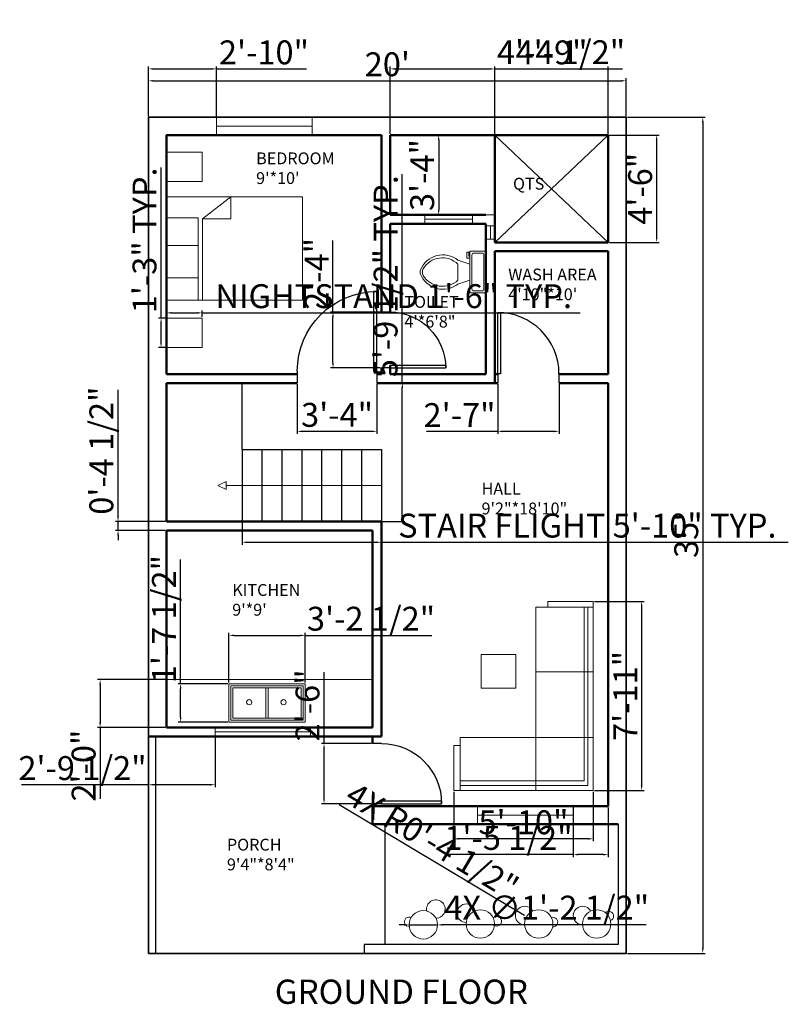
# Model space of a CAD drawing. Units: inches. Extents: x 2157 to 3060, y 2058 to 2553.
# Tile 1 of 2: x 2157 to 2543, y 2058 to 2553. Entities that reach past the tile are written whole.
import ezdxf

# ---------------------------------------------------------------- set-up
doc = ezdxf.new("R2010")
doc.units = ezdxf.units.IN
for name, color, linetype, lineweight in [('A-ANNO-DIMS', 2, 'Continuous', 18), ('A-ANNO-SYMB', 7, 'Continuous', 13), ('A-ANNO-TEXT', 7, 'Continuous', 35), ('A-AREA-IDEN', 7, 'Continuous', 18), ('A-FLOR', 7, 'Continuous', 25), ('A-FLOR-CASE', 32, 'Continuous', 20), ('A-FLOR-FIXT', 9, 'Continuous', 18), ('A-FLOR-STRS', 7, 'Continuous', 25), ('C-PROP', 7, 'Continuous', 35), ('DOOR', 2, 'Continuous', 25), ('FURNITURE', 32, 'Continuous', 18), ('L-PLNT', 3, 'Continuous', 18), ('WALL', 7, 'Continuous', 50), ('WINDOW', 130, 'Continuous', 18)]:
    doc.layers.add(name, color=color, linetype=linetype, lineweight=lineweight)
doc.styles.get("Standard").update_dxf_attribs({"font": 'arial.ttf'})
doc.dimstyles.new('ISO-25', dxfattribs={"dimtxt": 12, "dimasz": 2.5, "dimexe": 1.25, "dimexo": 0.625, "dimtad": 1, "dimdec": 0, "dimlunit": 4, "dimtxsty": 'Standard', "dimcen": 2.5, "dimadec": 0, "dimazin": 0, "dimtfac": 1, "dimtdec": 0, "dimtmove": 0, "dimatfit": 3, "dimfxl": 1, "dimarcsym": 0})

# ---------------------------------------------------------------- blocks, each defined once
blk = doc.blocks.new('*U2')
for p, q in [((0, 0), (0, -6)), ((40, 0), (40, -6))]:
    blk.add_line(p, q)
blk.add_lwpolyline([(0, 0), (0, 40), (1.75, 40), (1.75, 0)], close=True)
blk.add_arc((0, 0), 40, 0, 90)
blk = doc.blocks.new('*U4')
for p, q in [((9.5, -6), (9.5, -2)), ((-10, -8.5), (-8, -8.5)), ((-10, -9.5), (-10, -8.5)), ((-7, -9.5), (-10, -9.5)), ((-8, -8.5), (-8, -8)), ((-7, -8), (-7, -9.5)), ((-4, -8), (-6, -14)), ((4, -8), (6, -14)), ((4, -14), (-4, -14))]:
    blk.add_line(p, q)
blk.add_lwpolyline([(10.5, -8), (10.5, 0), (-10.5, 0), (-10.5, -8)], close=True)
for points in [[(-9.5, -2), (-9.5, -6)], [(8.5, -1), (-8.5, -1)], [(-8.5, -7), (8.5, -7)]]:
    blk.add_lwpolyline(points)
for centre, radius, start, end in [((-8.62, -1.88), 0.884, 81.8699, 188.1301), ((8.62, -1.88), 0.884, 351.8699, 98.1301), ((-8.62, -6.12), 0.884, 171.8699, 278.1301), ((8.62, -6.12), 0.884, 261.8699, 8.1301), ((3.52, -21.58), 12.17, 141.4691, 247.9714), ((4.2, -21.82), 11.33, 136.3677, 238.9468), ((-3.52, -21.58), 12.17, 292.0284, 38.5307), ((-4.2, -21.82), 11.33, 301.053, 43.6321), ((0, -27.88), 4, 245.7318, 294.2682), ((0, -29), 4, 254.8605, 285.1395)]:
    blk.add_arc(centre, radius, start, end)
blk = doc.blocks.new('*D5')
at = {"layer": 'A-ANNO-DIMS', "color": 0, "lineweight": -2, "transparency": 16777216}
for p, q in [((2222.04, 2504.59), (2222.04, 2523.53)), ((2462.04, 2504.59), (2462.04, 2523.53)), ((2224.54, 2522.28), (2459.54, 2522.28))]:
    blk.add_line(p, q, dxfattribs=at)
at = {"layer": 'A-ANNO-DIMS', "color": 0, "transparency": 16777216}
for points in [[(2224.54, 2522.7), (2224.54, 2521.86), (2222.04, 2522.28)], [(2459.54, 2522.7), (2459.54, 2521.86), (2462.04, 2522.28)]]:
    blk.add_solid(points, dxfattribs=at)
at = {"layer": 'Defpoints', "color": 0, "transparency": 16777216}
for p in [(2462.04, 2522.28), (2222.04, 2503.96), (2462.04, 2503.96)]:
    blk.add_point(p, dxfattribs=at)
at = {"layer": 'A-ANNO-DIMS', "color": 0, "transparency": 16777216, "insert": (2342.04, 2529.03), "char_height": 12, "attachment_point": 5}
blk.add_mtext("20'", dxfattribs=at)
blk = doc.blocks.new('*D6')
at = {"layer": 'A-ANNO-DIMS', "color": 0, "lineweight": -2, "transparency": 16777216}
for p, q in [((2462.67, 2503.96), (2501.77, 2503.96)), ((2500.52, 2501.46), (2500.52, 2086.46)), ((2462.67, 2083.96), (2501.77, 2083.96))]:
    blk.add_line(p, q, dxfattribs=at)
at = {"layer": 'A-ANNO-DIMS', "color": 0, "transparency": 16777216}
for points in [[(2500.1, 2501.46), (2500.94, 2501.46), (2500.52, 2503.96)], [(2500.1, 2086.46), (2500.94, 2086.46), (2500.52, 2083.96)]]:
    blk.add_solid(points, dxfattribs=at)
at = {"layer": 'Defpoints', "color": 0, "transparency": 16777216}
for p in [(2462.04, 2503.96), (2462.04, 2083.96), (2500.52, 2083.96)]:
    blk.add_point(p, dxfattribs=at)
at = {"layer": 'A-ANNO-DIMS', "color": 0, "transparency": 16777216, "insert": (2493.76, 2293.96), "char_height": 12, "attachment_point": 5, "rotation": 90}
blk.add_mtext("35'", dxfattribs=at)
blk = doc.blocks.new('BED-DOUBLE')
for p, q in [((18.2, 40.88), (32.33, 51.9)), ((32.33, 40.88), (32.33, 51.9)), ((18.2, 0), (18.2, 40.88)), ((18.2, 40.88), (32.33, 40.88)), ((0, 27.39), (15.88, 27.39)), ((0, 11.16), (15.88, 11.16))]:
    blk.add_line(p, q)
for points in [[(0, 0), (68.32, 0), (68.32, 51.9), (0, 51.9)], [(0, 0), (15.88, 0), (15.88, 41.3), (0, 41.3)]]:
    blk.add_lwpolyline(points, close=True)
blk = doc.blocks.new('NIGHTSTAND')
blk.add_lwpolyline([(0, 0), (17.99, 0), (17.99, 14.76), (0, 14.76)], close=True)
blk = doc.blocks.new('STAIR-FLIGHT')
for p, q in [((0, 36.14), (0, 69.5)), ((0, 36.14), (70, 36.14)), ((0, 36.14), (0, 0)), ((0, 36.14), (0, 0)), ((0, 36.14), (0, 0)), ((0, 36.14), (0, 0)), ((10, 36.14), (10, 0)), ((10, 36.14), (10, 0)), ((10, 36.14), (10, 0)), ((10, 36.14), (10, 0)), ((20, 36.14), (20, 0)), ((30, 36.14), (30, 0)), ((30, 36.14), (30, 0)), ((30, 36.14), (30, 0)), ((30, 36.14), (30, 0)), ((40, 36.14), (40, 0)), ((50, 36.14), (50, 0)), ((50, 36.14), (50, 0)), ((50, 36.14), (50, 0)), ((50, 36.14), (50, 0)), ((60, 36.14), (60, 0)), ((70, 36.14), (70, 0))]:
    blk.add_line(p, q)
blk = doc.blocks.new('STAIR-DIRECTION')
for p, q in [((4.17, 4), (0, 2)), ((0, 2), (4.17, 0)), ((4.17, 0), (4.17, 4)), ((82.21, 2), (4.17, 2)), ((4.17, 2), (4.17, 0))]:
    blk.add_line(p, q)
blk = doc.blocks.new('WIN-48IN-EXT')
for p, q in [((0, 4.5), (0, 9)), ((48, 4.5), (48, 9)), ((0, 4.5), (0, 0)), ((0, 4.5), (48, 4.5)), ((48, 4.5), (48, 0))]:
    blk.add_line(p, q)
blk = doc.blocks.new('OPEN-TO-SKY-MARK')
for p, q in [((57, 53.82), (0, 0)), ((57, 0), (0, 53.82))]:
    blk.add_line(p, q)
blk = doc.blocks.new('*D15')
at = {"layer": 'A-ANNO-DIMS', "color": 0, "lineweight": -2, "transparency": 16777216}
for p, q in [((2231.04, 2403.64), (2231.04, 2406.96)), ((2233.54, 2405.71), (2246.53, 2405.71)), ((2249.03, 2403.64), (2249.03, 2406.96)), ((2249.03, 2405.71), (2438.97, 2405.71))]:
    blk.add_line(p, q, dxfattribs=at)
at = {"layer": 'A-ANNO-DIMS', "color": 0, "transparency": 16777216}
for points in [[(2233.54, 2406.13), (2233.54, 2405.3), (2231.04, 2405.71)], [(2246.53, 2406.13), (2246.53, 2405.3), (2249.03, 2405.71)]]:
    blk.add_solid(points, dxfattribs=at)
at = {"layer": 'Defpoints', "color": 0, "transparency": 16777216}
for p in [(2249.03, 2405.71), (2231.04, 2403.02), (2249.03, 2403.02)]:
    blk.add_point(p, dxfattribs=at)
at = {"layer": 'A-ANNO-DIMS', "color": 0, "transparency": 16777216, "insert": (2345.25, 2412.54), "char_height": 12, "attachment_point": 5}
blk.add_mtext('NIGHTSTAND 1\'-6" TYP.', dxfattribs=at)
blk = doc.blocks.new('*D16')
at = {"layer": 'A-ANNO-DIMS', "color": 0, "lineweight": -2, "transparency": 16777216}
for p, q in [((2228.35, 2403.02), (2228.35, 2478.78)), ((2230.42, 2403.02), (2227.1, 2403.02)), ((2228.35, 2390.76), (2228.35, 2400.52)), ((2230.42, 2388.26), (2227.1, 2388.26))]:
    blk.add_line(p, q, dxfattribs=at)
at = {"layer": 'A-ANNO-DIMS', "color": 0, "transparency": 16777216}
for points in [[(2227.93, 2400.52), (2228.76, 2400.52), (2228.35, 2403.02)], [(2227.93, 2390.76), (2228.76, 2390.76), (2228.35, 2388.26)]]:
    blk.add_solid(points, dxfattribs=at)
at = {"layer": 'Defpoints', "color": 0, "transparency": 16777216}
for p in [(2228.35, 2403.02), (2231.04, 2403.02), (2231.04, 2388.26)]:
    blk.add_point(p, dxfattribs=at)
at = {"layer": 'A-ANNO-DIMS', "color": 0, "transparency": 16777216, "insert": (2221.59, 2442.15), "char_height": 12, "attachment_point": 5, "rotation": 90}
blk.add_mtext('1\'-3" TYP.', dxfattribs=at)
blk = doc.blocks.new('*D21')
at = {"layer": 'A-ANNO-DIMS', "color": 0, "lineweight": -2, "transparency": 16777216}
for p, q in [((2269.04, 2300.34), (2269.04, 2289.21)), ((2339.04, 2300.34), (2339.04, 2289.21)), ((2271.54, 2290.46), (2336.54, 2290.46)), ((2339.04, 2290.46), (2543.5, 2290.46))]:
    blk.add_line(p, q, dxfattribs=at)
at = {"layer": 'A-ANNO-DIMS', "color": 0, "transparency": 16777216}
for points in [[(2271.54, 2290.88), (2271.54, 2290.05), (2269.04, 2290.46)], [(2336.54, 2290.88), (2336.54, 2290.05), (2339.04, 2290.46)]]:
    blk.add_solid(points, dxfattribs=at)
at = {"layer": 'Defpoints', "color": 0, "transparency": 16777216}
for p in [(2269.04, 2300.96), (2339.04, 2300.96), (2339.04, 2290.46)]:
    blk.add_point(p, dxfattribs=at)
at = {"layer": 'A-ANNO-DIMS', "color": 0, "transparency": 16777216, "insert": (2442.52, 2297.29), "char_height": 12, "attachment_point": 5}
blk.add_mtext('STAIR FLIGHT 5\'-10" TYP.', dxfattribs=at)
blk = doc.blocks.new('*D22')
at = {"layer": 'A-ANNO-DIMS', "color": 0, "lineweight": -2, "transparency": 16777216}
for p, q in [((2349.54, 2370.46), (2349.54, 2475.32)), ((2339.67, 2370.46), (2350.79, 2370.46)), ((2349.54, 2303.46), (2349.54, 2367.96)), ((2339.67, 2300.96), (2350.79, 2300.96))]:
    blk.add_line(p, q, dxfattribs=at)
at = {"layer": 'A-ANNO-DIMS', "color": 0, "transparency": 16777216}
for points in [[(2349.13, 2367.96), (2349.96, 2367.96), (2349.54, 2370.46)], [(2349.13, 2303.46), (2349.96, 2303.46), (2349.54, 2300.96)]]:
    blk.add_solid(points, dxfattribs=at)
at = {"layer": 'Defpoints', "color": 0, "transparency": 16777216}
for p in [(2339.04, 2370.46), (2349.54, 2370.46), (2339.04, 2300.96)]:
    blk.add_point(p, dxfattribs=at)
at = {"layer": 'A-ANNO-DIMS', "color": 0, "transparency": 16777216, "insert": (2342.71, 2424.14), "char_height": 12, "attachment_point": 5, "rotation": 90}
blk.add_mtext('5\'-9 1/2" TYP.', dxfattribs=at)
blk = doc.blocks.new('*D23')
at = {"layer": 'A-ANNO-DIMS', "color": 0, "lineweight": -2, "transparency": 16777216}
for p, q in [((2396.04, 2495.59), (2396.04, 2529.51)), ((2398.54, 2528.26), (2450.54, 2528.26)), ((2453.04, 2495.59), (2453.04, 2529.51))]:
    blk.add_line(p, q, dxfattribs=at)
at = {"layer": 'A-ANNO-DIMS', "color": 0, "transparency": 16777216}
for points in [[(2398.54, 2528.68), (2398.54, 2527.85), (2396.04, 2528.26)], [(2450.54, 2528.68), (2450.54, 2527.85), (2453.04, 2528.26)]]:
    blk.add_solid(points, dxfattribs=at)
at = {"layer": 'Defpoints', "color": 0, "transparency": 16777216}
for p in [(2453.04, 2528.26), (2396.04, 2494.96), (2453.04, 2494.96)]:
    blk.add_point(p, dxfattribs=at)
at = {"layer": 'A-ANNO-DIMS', "color": 0, "transparency": 16777216, "insert": (2424.54, 2535.01), "char_height": 12, "attachment_point": 5}
blk.add_mtext('4\'-9"', dxfattribs=at)
blk = doc.blocks.new('*D24')
at = {"layer": 'A-ANNO-DIMS', "color": 0, "lineweight": -2, "transparency": 16777216}
for p, q in [((2453.67, 2494.96), (2478.59, 2494.96)), ((2477.34, 2492.46), (2477.34, 2443.64)), ((2453.67, 2441.14), (2478.59, 2441.14))]:
    blk.add_line(p, q, dxfattribs=at)
at = {"layer": 'A-ANNO-DIMS', "color": 0, "transparency": 16777216}
for points in [[(2476.93, 2492.46), (2477.76, 2492.46), (2477.34, 2494.96)], [(2476.93, 2443.64), (2477.76, 2443.64), (2477.34, 2441.14)]]:
    blk.add_solid(points, dxfattribs=at)
at = {"layer": 'Defpoints', "color": 0, "transparency": 16777216}
for p in [(2453.04, 2494.96), (2453.04, 2441.14), (2477.34, 2441.14)]:
    blk.add_point(p, dxfattribs=at)
at = {"layer": 'A-ANNO-DIMS', "color": 0, "transparency": 16777216, "insert": (2470.59, 2468.05), "char_height": 12, "attachment_point": 5, "rotation": 90}
blk.add_mtext('4\'-6"', dxfattribs=at)
blk = doc.blocks.new('*D27')
at = {"layer": 'A-ANNO-DIMS', "color": 0, "lineweight": -2, "transparency": 16777216}
for p, q in [((2310.24, 2189.36), (2310.24, 2225.21)), ((2333.92, 2189.36), (2308.99, 2189.36)), ((2310.24, 2161.64), (2310.24, 2186.86)), ((2333.92, 2159.14), (2308.99, 2159.14))]:
    blk.add_line(p, q, dxfattribs=at)
at = {"layer": 'A-ANNO-DIMS', "color": 0, "transparency": 16777216}
for points in [[(2309.83, 2186.86), (2310.66, 2186.86), (2310.24, 2189.36)], [(2309.83, 2161.64), (2310.66, 2161.64), (2310.24, 2159.14)]]:
    blk.add_solid(points, dxfattribs=at)
at = {"layer": 'Defpoints', "color": 0, "transparency": 16777216}
for p in [(2310.24, 2189.36), (2334.54, 2189.36), (2334.54, 2159.14)]:
    blk.add_point(p, dxfattribs=at)
at = {"layer": 'A-ANNO-DIMS', "color": 0, "transparency": 16777216, "insert": (2303.49, 2208.54), "char_height": 12, "attachment_point": 5, "rotation": 90}
blk.add_mtext('2\'-6"', dxfattribs=at)
blk = doc.blocks.new('*D29')
at = {"layer": 'A-ANNO-DIMS', "color": 0, "lineweight": -2, "transparency": 16777216}
for p, q in [((2230.42, 2221.46), (2196.49, 2221.46)), ((2197.74, 2218.96), (2197.74, 2199.96)), ((2230.42, 2197.46), (2196.49, 2197.46)), ((2197.74, 2197.46), (2197.74, 2161.61))]:
    blk.add_line(p, q, dxfattribs=at)
at = {"layer": 'A-ANNO-DIMS', "color": 0, "transparency": 16777216}
for points in [[(2197.33, 2218.96), (2198.16, 2218.96), (2197.74, 2221.46)], [(2197.33, 2199.96), (2198.16, 2199.96), (2197.74, 2197.46)]]:
    blk.add_solid(points, dxfattribs=at)
at = {"layer": 'Defpoints', "color": 0, "transparency": 16777216}
for p in [(2231.04, 2221.46), (2197.74, 2197.46), (2231.04, 2197.46)]:
    blk.add_point(p, dxfattribs=at)
at = {"layer": 'A-ANNO-DIMS', "color": 0, "transparency": 16777216, "insert": (2190.99, 2178.28), "char_height": 12, "attachment_point": 5, "rotation": 90}
blk.add_mtext('2\'-0"', dxfattribs=at)
blk = doc.blocks.new('*D30')
at = {"layer": 'A-ANNO-DIMS', "color": 0, "lineweight": -2, "transparency": 16777216}
for p, q in [((2222.04, 2504.59), (2222.04, 2529.51)), ((2224.54, 2528.26), (2253.72, 2528.26)), ((2256.22, 2504.59), (2256.22, 2529.51)), ((2256.22, 2528.26), (2301.4, 2528.26))]:
    blk.add_line(p, q, dxfattribs=at)
at = {"layer": 'A-ANNO-DIMS', "color": 0, "transparency": 16777216}
for points in [[(2224.54, 2528.68), (2224.54, 2527.85), (2222.04, 2528.26)], [(2253.72, 2528.68), (2253.72, 2527.85), (2256.22, 2528.26)]]:
    blk.add_solid(points, dxfattribs=at)
at = {"layer": 'Defpoints', "color": 0, "transparency": 16777216}
for p in [(2256.22, 2528.26), (2222.04, 2503.96), (2256.22, 2503.96)]:
    blk.add_point(p, dxfattribs=at)
at = {"layer": 'A-ANNO-DIMS', "color": 0, "transparency": 16777216, "insert": (2280.06, 2535.01), "char_height": 12, "attachment_point": 5}
blk.add_mtext('2\'-10"', dxfattribs=at)
blk = doc.blocks.new('*D32')
at = {"layer": 'A-ANNO-DIMS', "color": 0, "lineweight": -2, "transparency": 16777216}
for p, q in [((2222.04, 2192.34), (2222.04, 2167.41)), ((2255.49, 2192.34), (2255.49, 2167.41)), ((2222.04, 2168.66), (2158.23, 2168.66)), ((2252.99, 2168.66), (2224.54, 2168.66))]:
    blk.add_line(p, q, dxfattribs=at)
at = {"layer": 'A-ANNO-DIMS', "color": 0, "transparency": 16777216}
for points in [[(2224.54, 2169.08), (2224.54, 2168.25), (2222.04, 2168.66)], [(2252.99, 2169.08), (2252.99, 2168.25), (2255.49, 2168.66)]]:
    blk.add_solid(points, dxfattribs=at)
at = {"layer": 'Defpoints', "color": 0, "transparency": 16777216}
for p in [(2222.04, 2192.96), (2255.49, 2192.96), (2222.04, 2168.66)]:
    blk.add_point(p, dxfattribs=at)
at = {"layer": 'A-ANNO-DIMS', "color": 0, "transparency": 16777216, "insert": (2188.89, 2175.49), "char_height": 12, "attachment_point": 5}
blk.add_mtext('2\'-9 1/2"', dxfattribs=at)
blk = doc.blocks.new('*D33')
at = {"layer": 'A-ANNO-DIMS', "color": 0, "lineweight": -2, "transparency": 16777216}
for p, q in [((2435.4, 2157.26), (2435.4, 2132.33)), ((2453.04, 2157.26), (2453.04, 2132.33)), ((2435.4, 2133.58), (2372.92, 2133.58)), ((2450.54, 2133.58), (2437.9, 2133.58))]:
    blk.add_line(p, q, dxfattribs=at)
at = {"layer": 'A-ANNO-DIMS', "color": 0, "transparency": 16777216}
for points in [[(2437.9, 2134), (2437.9, 2133.16), (2435.4, 2133.58)], [(2450.54, 2134), (2450.54, 2133.16), (2453.04, 2133.58)]]:
    blk.add_solid(points, dxfattribs=at)
at = {"layer": 'Defpoints', "color": 0, "transparency": 16777216}
for p in [(2435.4, 2157.88), (2453.04, 2157.88), (2435.4, 2133.58)]:
    blk.add_point(p, dxfattribs=at)
at = {"layer": 'A-ANNO-DIMS', "color": 0, "transparency": 16777216, "insert": (2402.91, 2140.41), "char_height": 12, "attachment_point": 5}
blk.add_mtext('1\'-5 1/2"', dxfattribs=at)
blk = doc.blocks.new('*D36')
at = {"layer": 'A-ANNO-DIMS', "color": 0, "lineweight": -2, "transparency": 16777216}
for p, q in [((2296.79, 2369.84), (2296.79, 2344.91)), ((2336.79, 2369.84), (2336.79, 2344.91)), ((2334.29, 2346.16), (2299.29, 2346.16))]:
    blk.add_line(p, q, dxfattribs=at)
at = {"layer": 'A-ANNO-DIMS', "color": 0, "transparency": 16777216}
for points in [[(2299.29, 2346.58), (2299.29, 2345.75), (2296.79, 2346.16)], [(2334.29, 2346.58), (2334.29, 2345.75), (2336.79, 2346.16)]]:
    blk.add_solid(points, dxfattribs=at)
at = {"layer": 'Defpoints', "color": 0, "transparency": 16777216}
for p in [(2296.79, 2370.46), (2336.79, 2370.46), (2296.79, 2346.16)]:
    blk.add_point(p, dxfattribs=at)
at = {"layer": 'A-ANNO-DIMS', "color": 0, "transparency": 16777216, "insert": (2316.79, 2352.92), "char_height": 12, "attachment_point": 5}
blk.add_mtext('3\'-4"', dxfattribs=at)
blk = doc.blocks.new('*D37')
at = {"layer": 'A-ANNO-DIMS', "color": 0, "lineweight": -2, "transparency": 16777216}
for p, q in [((2397.49, 2369.84), (2397.49, 2344.91)), ((2428.29, 2369.84), (2428.29, 2344.91)), ((2397.49, 2346.16), (2361.64, 2346.16)), ((2425.79, 2346.16), (2399.99, 2346.16))]:
    blk.add_line(p, q, dxfattribs=at)
at = {"layer": 'A-ANNO-DIMS', "color": 0, "transparency": 16777216}
for points in [[(2399.99, 2346.58), (2399.99, 2345.75), (2397.49, 2346.16)], [(2425.79, 2346.58), (2425.79, 2345.75), (2428.29, 2346.16)]]:
    blk.add_solid(points, dxfattribs=at)
at = {"layer": 'Defpoints', "color": 0, "transparency": 16777216}
for p in [(2397.49, 2370.46), (2428.29, 2370.46), (2397.49, 2346.16)]:
    blk.add_point(p, dxfattribs=at)
at = {"layer": 'A-ANNO-DIMS', "color": 0, "transparency": 16777216, "insert": (2378.31, 2352.81), "char_height": 12, "attachment_point": 5}
blk.add_mtext('2\'-7"', dxfattribs=at)
blk = doc.blocks.new('*D38')
at = {"layer": 'A-ANNO-DIMS', "color": 0, "lineweight": -2, "transparency": 16777216}
for p, q in [((2314.74, 2406.14), (2314.74, 2441.99)), ((2338.42, 2406.14), (2313.49, 2406.14)), ((2314.74, 2380.53), (2314.74, 2403.64)), ((2338.42, 2378.03), (2313.49, 2378.03))]:
    blk.add_line(p, q, dxfattribs=at)
at = {"layer": 'A-ANNO-DIMS', "color": 0, "transparency": 16777216}
for points in [[(2314.33, 2403.64), (2315.16, 2403.64), (2314.74, 2406.14)], [(2314.33, 2380.53), (2315.16, 2380.53), (2314.74, 2378.03)]]:
    blk.add_solid(points, dxfattribs=at)
at = {"layer": 'Defpoints', "color": 0, "transparency": 16777216}
for p in [(2314.74, 2406.14), (2339.04, 2406.14), (2339.04, 2378.03)]:
    blk.add_point(p, dxfattribs=at)
at = {"layer": 'A-ANNO-DIMS', "color": 0, "transparency": 16777216, "insert": (2308.09, 2425.31), "char_height": 12, "attachment_point": 5, "rotation": 90}
blk.add_mtext('2\'-4"', dxfattribs=at)
blk = doc.blocks.new('*D41')
at = {"layer": 'A-ANNO-DIMS', "color": 0, "lineweight": -2, "transparency": 16777216}
for p, q in [((2375.38, 2165.16), (2375.38, 2140.24)), ((2445.5, 2165.16), (2445.5, 2140.24)), ((2443, 2141.49), (2377.88, 2141.49))]:
    blk.add_line(p, q, dxfattribs=at)
at = {"layer": 'A-ANNO-DIMS', "color": 0, "transparency": 16777216}
for points in [[(2377.88, 2141.91), (2377.88, 2141.07), (2375.38, 2141.49)], [(2443, 2141.91), (2443, 2141.07), (2445.5, 2141.49)]]:
    blk.add_solid(points, dxfattribs=at)
at = {"layer": 'Defpoints', "color": 0, "transparency": 16777216}
for p in [(2375.38, 2165.79), (2445.5, 2165.79), (2375.38, 2141.49)]:
    blk.add_point(p, dxfattribs=at)
at = {"layer": 'A-ANNO-DIMS', "color": 0, "transparency": 16777216, "insert": (2410.44, 2148.24), "char_height": 12, "attachment_point": 5}
blk.add_mtext('5\'-10"', dxfattribs=at)
blk = doc.blocks.new('*D42')
at = {"layer": 'A-ANNO-DIMS', "color": 0, "lineweight": -2, "transparency": 16777216}
for p, q in [((2446.13, 2260.8), (2471.05, 2260.8)), ((2469.8, 2258.3), (2469.8, 2168.29)), ((2446.13, 2165.79), (2471.05, 2165.79))]:
    blk.add_line(p, q, dxfattribs=at)
at = {"layer": 'A-ANNO-DIMS', "color": 0, "transparency": 16777216}
for points in [[(2469.39, 2258.3), (2470.22, 2258.3), (2469.8, 2260.8)], [(2469.39, 2168.29), (2470.22, 2168.29), (2469.8, 2165.79)]]:
    blk.add_solid(points, dxfattribs=at)
at = {"layer": 'Defpoints', "color": 0, "transparency": 16777216}
for p in [(2445.5, 2260.8), (2445.5, 2165.79), (2469.8, 2165.79)]:
    blk.add_point(p, dxfattribs=at)
at = {"layer": 'A-ANNO-DIMS', "color": 0, "transparency": 16777216, "insert": (2463.15, 2213.29), "char_height": 12, "attachment_point": 5, "rotation": 90}
blk.add_mtext('7\'-11"', dxfattribs=at)
blk = doc.blocks.new('*D43')
at = {"layer": 'A-ANNO-DIMS', "color": 0, "lineweight": -2, "transparency": 16777216}
for p, q in [((2262.49, 2220.01), (2262.49, 2244.94)), ((2264.99, 2243.69), (2298.31, 2243.69)), ((2300.81, 2220.01), (2300.81, 2244.94)), ((2300.81, 2243.69), (2364.41, 2243.69))]:
    blk.add_line(p, q, dxfattribs=at)
at = {"layer": 'A-ANNO-DIMS', "color": 0, "transparency": 16777216}
for points in [[(2264.99, 2244.1), (2264.99, 2243.27), (2262.49, 2243.69)], [(2298.31, 2244.1), (2298.31, 2243.27), (2300.81, 2243.69)]]:
    blk.add_solid(points, dxfattribs=at)
at = {"layer": 'Defpoints', "color": 0, "transparency": 16777216}
for p in [(2300.81, 2243.69), (2262.49, 2219.39), (2300.81, 2219.39)]:
    blk.add_point(p, dxfattribs=at)
at = {"layer": 'A-ANNO-DIMS', "color": 0, "transparency": 16777216, "insert": (2333.86, 2250.52), "char_height": 12, "attachment_point": 5}
blk.add_mtext('3\'-2 1/2"', dxfattribs=at)
blk = doc.blocks.new('*D44')
at = {"layer": 'A-ANNO-DIMS', "color": 0, "lineweight": -2, "transparency": 16777216}
for p, q in [((2238.19, 2219.39), (2238.19, 2281.87)), ((2261.87, 2219.39), (2236.94, 2219.39)), ((2238.19, 2202.61), (2238.19, 2216.89)), ((2261.87, 2200.11), (2236.94, 2200.11))]:
    blk.add_line(p, q, dxfattribs=at)
at = {"layer": 'A-ANNO-DIMS', "color": 0, "transparency": 16777216}
for points in [[(2237.78, 2216.89), (2238.61, 2216.89), (2238.19, 2219.39)], [(2237.78, 2202.61), (2238.61, 2202.61), (2238.19, 2200.11)]]:
    blk.add_solid(points, dxfattribs=at)
at = {"layer": 'Defpoints', "color": 0, "transparency": 16777216}
for p in [(2238.19, 2219.39), (2262.49, 2219.39), (2262.49, 2200.11)]:
    blk.add_point(p, dxfattribs=at)
at = {"layer": 'A-ANNO-DIMS', "color": 0, "transparency": 16777216, "insert": (2231.36, 2251.88), "char_height": 12, "attachment_point": 5, "rotation": 90}
blk.add_mtext('1\'-7 1/2"', dxfattribs=at)
blk = doc.blocks.new('*D47')
at = {"layer": 'A-ANNO-DIMS', "color": 0, "lineweight": -2, "transparency": 16777216}
for p, q in [((2343.54, 2495.59), (2343.54, 2529.51)), ((2346.04, 2528.26), (2393.54, 2528.26)), ((2396.04, 2495.59), (2396.04, 2529.51)), ((2396.04, 2528.26), (2460.14, 2528.26))]:
    blk.add_line(p, q, dxfattribs=at)
at = {"layer": 'A-ANNO-DIMS', "color": 0, "transparency": 16777216}
for points in [[(2346.04, 2528.68), (2346.04, 2527.85), (2343.54, 2528.26)], [(2393.54, 2528.68), (2393.54, 2527.85), (2396.04, 2528.26)]]:
    blk.add_solid(points, dxfattribs=at)
at = {"layer": 'Defpoints', "color": 0, "transparency": 16777216}
for p in [(2396.04, 2528.26), (2343.54, 2494.96), (2396.04, 2494.96)]:
    blk.add_point(p, dxfattribs=at)
at = {"layer": 'A-ANNO-DIMS', "color": 0, "transparency": 16777216, "insert": (2429.34, 2535.09), "char_height": 12, "attachment_point": 5}
blk.add_mtext('4\'-4 1/2"', dxfattribs=at)
blk = doc.blocks.new('*D48')
at = {"layer": 'A-ANNO-DIMS', "color": 0, "lineweight": -2, "transparency": 16777216}
for p, q in [((2344.17, 2494.96), (2369.09, 2494.96)), ((2367.84, 2492.46), (2367.84, 2457.46)), ((2344.17, 2454.96), (2369.09, 2454.96))]:
    blk.add_line(p, q, dxfattribs=at)
at = {"layer": 'A-ANNO-DIMS', "color": 0, "transparency": 16777216}
for points in [[(2367.43, 2492.46), (2368.26, 2492.46), (2367.84, 2494.96)], [(2367.43, 2457.46), (2368.26, 2457.46), (2367.84, 2454.96)]]:
    blk.add_solid(points, dxfattribs=at)
at = {"layer": 'Defpoints', "color": 0, "transparency": 16777216}
for p in [(2343.54, 2494.96), (2343.54, 2454.96), (2367.84, 2454.96)]:
    blk.add_point(p, dxfattribs=at)
at = {"layer": 'A-ANNO-DIMS', "color": 0, "transparency": 16777216, "insert": (2361.09, 2474.96), "char_height": 12, "attachment_point": 5, "rotation": 90}
blk.add_mtext('3\'-4"', dxfattribs=at)
blk = doc.blocks.new('*D52')
at = {"layer": 'A-ANNO-DIMS', "color": 0, "lineweight": -2, "transparency": 16777216}
for p, q in [((2206.74, 2303.46), (2206.74, 2367.07)), ((2230.42, 2300.96), (2205.49, 2300.96)), ((2206.74, 2296.46), (2206.74, 2300.96)), ((2230.42, 2296.46), (2205.49, 2296.46)), ((2206.74, 2293.96), (2206.74, 2291.46))]:
    blk.add_line(p, q, dxfattribs=at)
at = {"layer": 'A-ANNO-DIMS', "color": 0, "transparency": 16777216}
for points in [[(2206.33, 2303.46), (2207.16, 2303.46), (2206.74, 2300.96)], [(2206.33, 2293.96), (2207.16, 2293.96), (2206.74, 2296.46)]]:
    blk.add_solid(points, dxfattribs=at)
at = {"layer": 'Defpoints', "color": 0, "transparency": 16777216}
for p in [(2206.74, 2300.96), (2231.04, 2300.96), (2231.04, 2296.46)]:
    blk.add_point(p, dxfattribs=at)
at = {"layer": 'A-ANNO-DIMS', "color": 0, "transparency": 16777216, "insert": (2199.91, 2336.52), "char_height": 12, "attachment_point": 5, "rotation": 90}
blk.add_mtext('0\'-4 1/2"', dxfattribs=at)
blk = doc.blocks.new('*D53')
at = {"layer": 'A-ANNO-DIMS', "color": 0, "lineweight": -2, "transparency": 16777216}
for p, q in [((2350.45, 2098.29), (2347.95, 2098.29)), ((2352.95, 2098.29), (2367.23, 2098.29)), ((2472.02, 2098.29), (2369.73, 2098.29))]:
    blk.add_line(p, q, dxfattribs=at)
at = {"layer": 'A-ANNO-DIMS', "color": 0, "transparency": 16777216}
for points in [[(2350.45, 2098.71), (2350.45, 2097.87), (2352.95, 2098.29)], [(2369.73, 2098.71), (2369.73, 2097.87), (2367.23, 2098.29)]]:
    blk.add_solid(points, dxfattribs=at)
at = {"layer": 'Defpoints', "color": 0, "transparency": 16777216}
for p in [(2352.95, 2098.29), (2367.23, 2098.29)]:
    blk.add_point(p, dxfattribs=at)
at = {"layer": 'A-ANNO-DIMS', "color": 0, "transparency": 16777216, "insert": (2422.13, 2105.38), "char_height": 12, "attachment_point": 5, "rotation": 359.9997}
blk.add_mtext('4X ∅1\'-2 1/2"', dxfattribs=at)
blk = doc.blocks.new('*D54')
at = {"layer": 'A-ANNO-DIMS', "color": 0, "lineweight": -2, "transparency": 16777216}
for p, q in [((2317.87, 2158.67), (2404.87, 2106.65)), ((2411, 2102.98), (2407.01, 2105.37))]:
    blk.add_line(p, q, dxfattribs=at)
at = {"layer": 'A-ANNO-DIMS', "color": 0, "transparency": 16777216}
blk.add_solid([(2405.08, 2107.01), (2404.65, 2106.29), (2407.01, 2105.37)], dxfattribs=at)
at = {"layer": 'Defpoints', "color": 0, "transparency": 16777216}
for p in [(2407.01, 2105.37), (2411, 2102.98)]:
    blk.add_point(p, dxfattribs=at)
at = {"layer": 'A-ANNO-DIMS', "color": 0, "transparency": 16777216, "insert": (2363.8, 2139.16), "char_height": 12, "attachment_point": 5, "rotation": 329.124}
blk.add_mtext('4X R0\'-4 1/2"', dxfattribs=at)

msp = doc.modelspace()

# ---------------------------------------------------------------- linework, layer by layer
at = {"layer": 'A-FLOR'}
for p, q in [((2225.53, 2192.96), (2225.53, 2083.96)), ((2340.74, 2148.88), (2340.74, 2092.96)), ((2457.93, 2148.88), (2457.93, 2088.42)), ((2340.74, 2092.96), (2340.74, 2088.42)), ((2341.27, 2088.42), (2330.37, 2088.42)), ((2330.37, 2088.42), (2330.37, 2083.96)), ((2457.93, 2088.42), (2340.74, 2088.42))]:
    msp.add_line(p, q, dxfattribs=at)
at = {"layer": 'A-FLOR-CASE'}
for p, q in [((2231.04, 2197.46), (2231.04, 2221.46)), ((2231.04, 2221.46), (2334.54, 2221.46))]:
    msp.add_line(p, q, dxfattribs=at)
at = {"layer": 'A-FLOR-FIXT'}
for p, q in [((2281.08, 2217.39), (2281.08, 2202.11)), ((2282.2, 2202.11), (2282.2, 2217.39))]:
    msp.add_line(p, q, dxfattribs=at)
for points in [[(2262.49, 2219.39), (2300.81, 2219.39), (2300.81, 2200.11), (2262.49, 2200.11)], [(2263.49, 2218.39), (2299.81, 2218.39), (2299.81, 2201.11), (2263.49, 2201.11)], [(2264.49, 2217.39), (2298.81, 2217.39), (2298.81, 2202.11), (2264.49, 2202.11)]]:
    msp.add_lwpolyline(points, close=True, dxfattribs=at)
for centre in [(2272.66, 2210.13), (2289.91, 2210.13)]:
    msp.add_circle(centre, 1.32, dxfattribs=at)
at = {"layer": 'C-PROP'}
msp.add_lwpolyline([(2222.04, 2083.96), (2462.04, 2083.96), (2462.04, 2503.96), (2222.04, 2503.96)], close=True, dxfattribs=at)
at = {"layer": 'FURNITURE'}
for p, q in [((2422.64, 2257.82), (2422.64, 2260.8)), ((2422.64, 2260.8), (2445.5, 2260.8)), ((2445.5, 2260.8), (2445.5, 2256.85)), ((2441.01, 2257.82), (2441.01, 2170.59)), ((2442.7, 2257.82), (2442.7, 2168.27)), ((2416.6, 2225.42), (2445.5, 2225.42)), ((2378.61, 2188.45), (2375.38, 2188.45)), ((2375.38, 2188.45), (2375.38, 2165.79)), ((2441.01, 2170.59), (2378.61, 2170.59)), ((2442.7, 2168.27), (2378.61, 2168.27)), ((2375.38, 2165.79), (2380.51, 2165.79))]:
    msp.add_line(p, q, dxfattribs=at)
for points in [[(2445.5, 2165.79), (2416.6, 2165.79), (2416.6, 2257.82), (2445.5, 2257.82)], [(2389.24, 2234.02), (2406.52, 2234.02), (2406.52, 2217.17), (2389.24, 2217.17)], [(2445.5, 2165.79), (2378.61, 2165.79), (2378.61, 2192.32), (2445.5, 2192.32)]]:
    msp.add_lwpolyline(points, close=True, dxfattribs=at)
at = {"layer": 'L-PLNT'}
for centre in [(2360.09, 2098.29), (2388.79, 2098.72), (2418.13, 2098.72), (2447.25, 2098.72)]:
    msp.add_circle(centre, 7.14, dxfattribs=at)
for centre, radius, start, end in [((2366.43, 2106.22), 4.65, 270, 192.7389), ((2381.69, 2104.13), 4.65, 15.3254, 270), ((2411, 2102.98), 4.65, 28.2451, 270), ((2440.13, 2102.95), 4.65, 28.6334, 270), ((2353.08, 2099.83), 2.41, 66.8988, 268.311), ((2396.98, 2100.05), 2.41, 242.6654, 135.7072), ((2453.33, 2102.68), 2.41, 290.7865, 135.4739), ((2425.23, 2099.68), 2.41, 267.408, 108.0305)]:
    msp.add_arc(centre, radius, start, end, dxfattribs=at)
at = {"layer": 'WALL'}
for p, q in [((2231.04, 2494.96), (2339.04, 2494.96)), ((2339.04, 2494.96), (2339.04, 2406.14)), ((2343.54, 2494.96), (2387.04, 2494.96)), ((2343.54, 2494.96), (2343.54, 2454.96)), ((2396.04, 2494.96), (2396.04, 2441.14)), ((2453.04, 2441.14), (2453.04, 2494.96)), ((2391.54, 2454.96), (2343.54, 2454.96)), ((2391.54, 2450.46), (2343.54, 2450.46)), ((2343.54, 2450.46), (2343.54, 2406.13)), ((2391.54, 2450.46), (2391.54, 2374.96)), ((2396.04, 2441.14), (2453.04, 2441.14)), ((2396.04, 2370.46), (2396.04, 2436.64)), ((2396.04, 2436.64), (2453.04, 2436.64)), ((2396.04, 2436.64), (2396.04, 2370.46)), ((2453.04, 2374.96), (2453.04, 2436.64)), ((2343.54, 2379.26), (2343.54, 2374.96)), ((2296.79, 2374.96), (2231.04, 2374.96)), ((2339.04, 2374.96), (2336.79, 2374.96)), ((2339.04, 2378.03), (2339.04, 2374.96)), ((2391.54, 2374.96), (2343.54, 2374.96)), ((2396.04, 2374.96), (2397.49, 2374.96)), ((2428.29, 2374.96), (2453.04, 2374.96)), ((2296.79, 2370.46), (2231.04, 2370.46)), ((2343.54, 2370.46), (2336.79, 2370.46)), ((2396.04, 2370.46), (2339.04, 2370.46)), ((2396.04, 2370.46), (2397.49, 2370.46)), ((2428.29, 2370.46), (2453.04, 2370.46)), ((2231.04, 2300.96), (2339.04, 2300.96)), ((2339.04, 2300.96), (2339.04, 2192.96)), ((2231.04, 2197.46), (2231.04, 2296.46)), ((2231.04, 2296.46), (2334.54, 2296.46)), ((2334.54, 2296.46), (2334.54, 2197.46)), ((2231.04, 2197.46), (2334.54, 2197.46)), ((2231.04, 2192.96), (2222.04, 2192.96)), ((2231.04, 2192.96), (2339.04, 2192.96)), ((2334.54, 2192.96), (2334.54, 2189.36)), ((2334.54, 2159.14), (2334.54, 2148.88)), ((2343.04, 2157.88), (2334.54, 2157.88)), ((2343.04, 2157.88), (2453.04, 2157.88)), ((2334.54, 2148.88), (2343.04, 2148.88)), ((2343.04, 2148.88), (2453.04, 2148.88)), ((2453.04, 2148.88), (2457.93, 2148.88))]:
    msp.add_line(p, q, dxfattribs=at)
for points in [[(2339.04, 2494.96), (2231.04, 2494.96), (2231.04, 2374.96)], [(2453.04, 2441.14), (2453.04, 2494.96), (2343.54, 2494.96)], [(2453.04, 2374.96), (2453.04, 2436.64)], [(2231.04, 2370.46), (2231.04, 2300.96)], [(2453.04, 2157.88), (2453.04, 2370.46)], [(2231.04, 2296.46), (2231.04, 2197.46)]]:
    msp.add_lwpolyline(points, dxfattribs=at)
at = {"layer": 'WINDOW'}
for p, q in [((2360.85, 2454.96), (2360.85, 2450.46)), ((2384.85, 2454.96), (2384.85, 2450.46)), ((2391.54, 2454.96), (2396.04, 2454.96)), ((2360.85, 2452.71), (2384.85, 2452.71)), ((2391.54, 2449.35), (2396.04, 2449.35)), ((2393.79, 2449.35), (2393.79, 2442.69)), ((2396.04, 2441.14), (2396.04, 2450.46)), ((2391.54, 2442.69), (2396.04, 2442.69)), ((2255.49, 2197.46), (2255.49, 2192.96)), ((2303.49, 2197.46), (2303.49, 2192.96)), ((2255.49, 2195.21), (2303.49, 2195.21))]:
    msp.add_line(p, q, dxfattribs=at)

# ---------------------------------------------------------------- block references
at = {"layer": 'A-ANNO-SYMB', "rotation": 180}
msp.add_blockref('OPEN-TO-SKY-MARK', (2453.04, 2494.96), dxfattribs=at)
at = {"layer": 'A-ANNO-SYMB'}
msp.add_blockref('STAIR-DIRECTION', (2256.83, 2317.04), dxfattribs=at)
at = {"layer": 'A-FLOR-FIXT', "rotation": 270}
msp.add_blockref('*U4', (2391.54, 2426.21), dxfattribs=at)
at = {"layer": 'A-FLOR-STRS'}
msp.add_blockref('STAIR-FLIGHT', (2269.04, 2300.96), dxfattribs=at)
at = {"layer": 'DOOR', "xscale": -1}
msp.add_blockref('*U2', (2336.79, 2376.46), dxfattribs=at)
at = {"layer": 'DOOR', "rotation": 270}
for p, xscale, yscale, zscale in [((2343.26, 2378.03), -0.702626671553409, 0.702626671553409, 0.702626671553409), ((2339.08, 2159.14), -0.7555564324099674, 0.7555564324099674, 0.7555564324099674)]:
    msp.add_blockref('*U2', p, dxfattribs=dict(at, xscale=xscale, yscale=yscale, zscale=zscale))
at = {"layer": 'DOOR', "xscale": 0.7698686144923367, "yscale": 0.7698686144923367, "zscale": 0.7698686144923367}
msp.add_blockref('*U2', (2397.49, 2375.08), dxfattribs=at)
at = {"layer": 'FURNITURE'}
for name, p in [('NIGHTSTAND', (2231.04, 2471.73)), ('BED-DOUBLE', (2231.04, 2412.1)), ('NIGHTSTAND', (2231.04, 2388.26))]:
    msp.add_blockref(name, p, dxfattribs=at)
at = {"layer": 'WINDOW'}
for p in [(2256.22, 2494.96), (2387.4, 2148.88)]:
    msp.add_blockref('WIN-48IN-EXT', p, dxfattribs=at)

# ---------------------------------------------------------------- texts
at = {"layer": 'A-ANNO-TEXT', "insert": (2285.49, 2070.8), "char_height": 12.2084, "attachment_point": 1}
msp.add_mtext_dynamic_manual_height_columns('GROUND FLOOR', width=597.5375, gutter_width=61.04, heights=[0], dxfattribs=at)
at = {"layer": 'A-AREA-IDEN', "attachment_point": 1}
for s, insert, char_height in [("BEDROOM\\P9'*10'", (2276.11, 2486.31), 5.949), ('QTS', (2405.18, 2473.56), 5.949), ('WASH AREA\\P4\'10"*10\'', (2402.78, 2427.93), 5.949), ('TOILET\\P4\'*6\'8"', (2350.6, 2414.21), 5.949), ('HALL\\P9\'2"*18\'10"', (2389.38, 2320.34), 5.9493), ("KITCHEN\\P9'*9'", (2264.12, 2269.47), 5.949), ('PORCH\\P9\'4"*8\'4"', (2261.46, 2141.53), 5.949)]:
    msp.add_mtext_dynamic_manual_height_columns(s, width=65.8339, gutter_width=29.75, heights=[0], dxfattribs=dict(at, insert=insert, char_height=char_height))

# ---------------------------------------------------------------- dimensions: what is measured, and where the dimension line sits
at = {"layer": 'A-ANNO-DIMS'}
for base, p1, p2, override, picture, middle in [((2396.04, 2528.26), (2343.54, 2494.96), (2396.04, 2494.96), {"dimdec": 1, "dimlfac": 1, "dimrnd": 0, "dimzin": 1, "dimdsep": 46, "dimlunit": 4, "dimfrac": 2}, '*D47', (2429.34, 2535.09)), ((2256.22, 2528.26), (2222.04, 2503.96), (2256.22, 2503.96), {"dimdec": 1, "dimlfac": 1, "dimrnd": 0, "dimzin": 1, "dimdsep": 46, "dimlunit": 4, "dimfrac": 2}, '*D30', (2280.06, 2535.01)), ((2453.04, 2528.26), (2396.04, 2494.96), (2453.04, 2494.96), {"dimdec": 1, "dimlfac": 1, "dimrnd": 0, "dimzin": 1, "dimdsep": 46, "dimlunit": 4, "dimfrac": 2}, '*D23', (2424.54, 2535.01)), ((2462.04, 2522.28), (2222.04, 2503.96), (2462.04, 2503.96), {"dimclrd": 0, "dimclre": 0, "dimclrt": 0}, '*D5', (2342.04, 2529.03)), ((2300.81, 2243.69), (2262.49, 2219.39), (2300.81, 2219.39), {"dimdec": 1, "dimlfac": 1, "dimrnd": 0, "dimzin": 1, "dimdsep": 46, "dimlunit": 4, "dimfrac": 2}, '*D43', (2333.86, 2250.52))]:
    dim = msp.add_linear_dim(base=base, p1=p1, p2=p2, dimstyle='ISO-25', override=override, dxfattribs=at)
    dim.commit()
    dim.dimension.update_dxf_attribs({"geometry": picture, "text_midpoint": middle})
for base, p1, p2, angle, override, picture, middle in [((2500.52, 2083.96), (2462.04, 2503.96), (2462.04, 2083.96), 90, {"dimclrd": 0, "dimclre": 0, "dimclrt": 0}, '*D6', (2493.76, 2293.96)), ((2367.84, 2454.96), (2343.54, 2494.96), (2343.54, 2454.96), 270, {"dimdec": 1, "dimlfac": 1, "dimrnd": 0, "dimzin": 1, "dimdsep": 46, "dimlunit": 4, "dimfrac": 2}, '*D48', (2361.09, 2474.96)), ((2477.34, 2441.14), (2453.04, 2494.96), (2453.04, 2441.14), 270, {"dimdec": 1, "dimlfac": 1, "dimrnd": 0, "dimzin": 1, "dimdsep": 46, "dimlunit": 4, "dimfrac": 2}, '*D24', (2470.59, 2468.05)), ((2314.74, 2406.14), (2339.04, 2378.03), (2339.04, 2406.14), 90, {"dimdec": 1, "dimlfac": 1, "dimrnd": 0, "dimzin": 1, "dimdsep": 46, "dimlunit": 4, "dimfrac": 2}, '*D38', (2308.09, 2425.31)), ((2296.79, 2346.16), (2336.79, 2370.46), (2296.79, 2370.46), 180, {"dimdec": 1, "dimlfac": 1, "dimrnd": 0, "dimzin": 1, "dimdsep": 46, "dimlunit": 4, "dimfrac": 2}, '*D36', (2316.79, 2352.92)), ((2397.49, 2346.16), (2428.29, 2370.46), (2397.49, 2370.46), 180, {"dimdec": 1, "dimlfac": 1, "dimrnd": 0, "dimzin": 1, "dimdsep": 46, "dimlunit": 4, "dimfrac": 2}, '*D37', (2378.31, 2352.81)), ((2206.74, 2300.96), (2231.04, 2296.46), (2231.04, 2300.96), 90, {"dimdec": 1, "dimlfac": 1, "dimrnd": 0, "dimzin": 1, "dimdsep": 46, "dimlunit": 4, "dimfrac": 2}, '*D52', (2199.91, 2336.52)), ((2238.19, 2219.39), (2262.49, 2200.11), (2262.49, 2219.39), 90, {"dimdec": 1, "dimlfac": 1, "dimrnd": 0, "dimzin": 1, "dimdsep": 46, "dimlunit": 4, "dimfrac": 2}, '*D44', (2231.36, 2251.88)), ((2469.8, 2165.79), (2445.5, 2260.8), (2445.5, 2165.79), 270, {"dimdec": 1, "dimlfac": 1, "dimrnd": 0, "dimzin": 1, "dimdsep": 46, "dimlunit": 4, "dimfrac": 2}, '*D42', (2463.15, 2213.29)), ((2310.24, 2189.36), (2334.54, 2159.14), (2334.54, 2189.36), 90, {"dimdec": 1, "dimlfac": 1, "dimrnd": 0, "dimzin": 1, "dimdsep": 46, "dimlunit": 4, "dimfrac": 2}, '*D27', (2303.49, 2208.54)), ((2197.74, 2197.46), (2231.04, 2221.46), (2231.04, 2197.46), 90, {"dimdec": 1, "dimlfac": 1, "dimrnd": 0, "dimzin": 1, "dimdsep": 46, "dimlunit": 4, "dimfrac": 2}, '*D29', (2190.99, 2178.28)), ((2222.0444, 2168.6617), (2255.4863, 2192.9617), (2222.0444, 2192.9617), 180, {"dimdec": 1, "dimlfac": 1, "dimrnd": 0, "dimzin": 1, "dimdsep": 46, "dimlunit": 4, "dimfrac": 2}, '*D32', (2188.8866, 2175.4913)), ((2375.38, 2141.49), (2445.5, 2165.79), (2375.38, 2165.79), 180, {"dimdec": 1, "dimlfac": 1, "dimrnd": 0, "dimzin": 1, "dimdsep": 46, "dimlunit": 4, "dimfrac": 2}, '*D41', (2410.44, 2148.24)), ((2435.4, 2133.58), (2453.04, 2157.88), (2435.4, 2157.88), 180, {"dimdec": 1, "dimlfac": 1, "dimrnd": 0, "dimzin": 1, "dimdsep": 46, "dimlunit": 4, "dimfrac": 2}, '*D33', (2402.91, 2140.41))]:
    dim = msp.add_linear_dim(base=base, p1=p1, p2=p2, angle=angle, dimstyle='ISO-25', override=override, dxfattribs=at)
    dim.commit()
    dim.dimension.update_dxf_attribs({"geometry": picture, "text_midpoint": middle})
for base, p1, p2, picture, middle in [((2228.35, 2403.02), (2231.04, 2388.26), (2231.04, 2403.02), '*D16', (2221.59, 2442.15)), ((2349.54, 2370.46), (2339.04, 2300.96), (2339.04, 2370.46), '*D22', (2342.71, 2424.14))]:
    dim = msp.add_linear_dim(base=base, p1=p1, p2=p2, angle=90, text='<> TYP.', dimstyle='ISO-25', override={"dimdec": 1, "dimlfac": 1, "dimrnd": 0, "dimzin": 1, "dimdsep": 46, "dimlunit": 4, "dimfrac": 2}, dxfattribs=at)
    dim.commit()
    dim.dimension.update_dxf_attribs({"geometry": picture, "text_midpoint": middle})
for base, p1, p2, text, picture, middle in [((2249.03, 2405.71), (2231.04, 2403.02), (2249.03, 2403.02), 'NIGHTSTAND <> TYP.', '*D15', (2345.25, 2412.54)), ((2339.04, 2290.46), (2269.04, 2300.96), (2339.04, 2300.96), 'STAIR FLIGHT <> TYP.', '*D21', (2442.52, 2297.29))]:
    dim = msp.add_linear_dim(base=base, p1=p1, p2=p2, text=text, dimstyle='ISO-25', override={"dimdec": 1, "dimlfac": 1, "dimrnd": 0, "dimzin": 1, "dimdsep": 46, "dimlunit": 4, "dimfrac": 2}, dxfattribs=at)
    dim.commit()
    dim.dimension.update_dxf_attribs({"geometry": picture, "text_midpoint": middle})
dim = msp.add_radius_dim(center=(2411.0005, 2102.9822), mpoint=(2407.0122, 2105.3669), text='4X <>', dimstyle='ISO-25', override={"dimdec": 1, "dimlfac": 1, "dimrnd": 0, "dimzin": 1, "dimdsep": 46, "dimlunit": 4, "dimfrac": 2}, dxfattribs=at)
dim.commit()
dim.dimension.update_dxf_attribs({"geometry": '*D54', "text_midpoint": (2363.7997, 2139.1618)})
dim = msp.add_diameter_dim_2p(p1=(2352.95, 2098.29), p2=(2367.23, 2098.29), text='4X <>', dimstyle='ISO-25', override={"dimdec": 1, "dimlfac": 1, "dimrnd": 0, "dimzin": 1, "dimdsep": 46, "dimlunit": 4, "dimfrac": 2}, dxfattribs=at)
dim.commit()
dim.dimension.update_dxf_attribs({"geometry": '*D53', "text_midpoint": (2422.13, 2098.29), "dimtype": 163})

doc.saveas('drawing.dxf')
